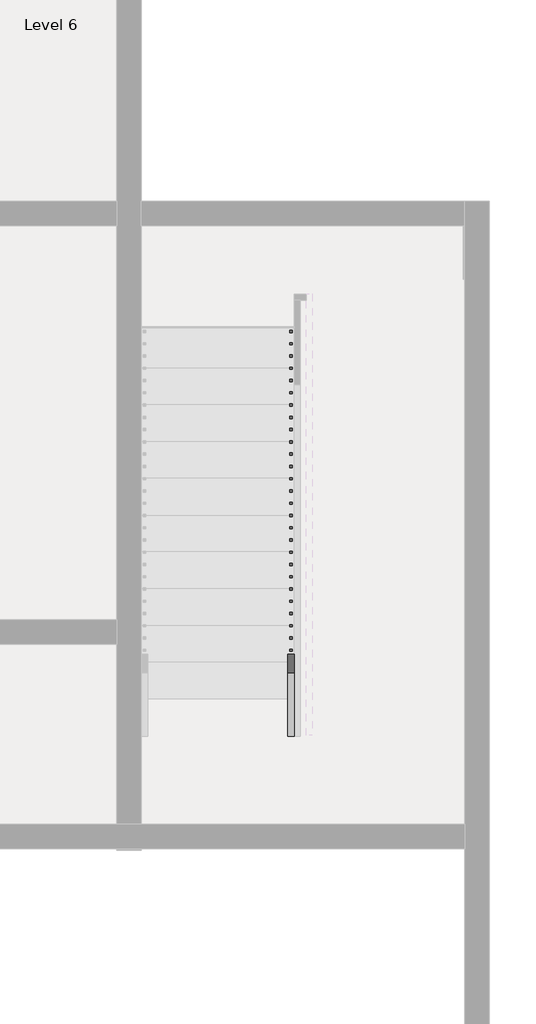
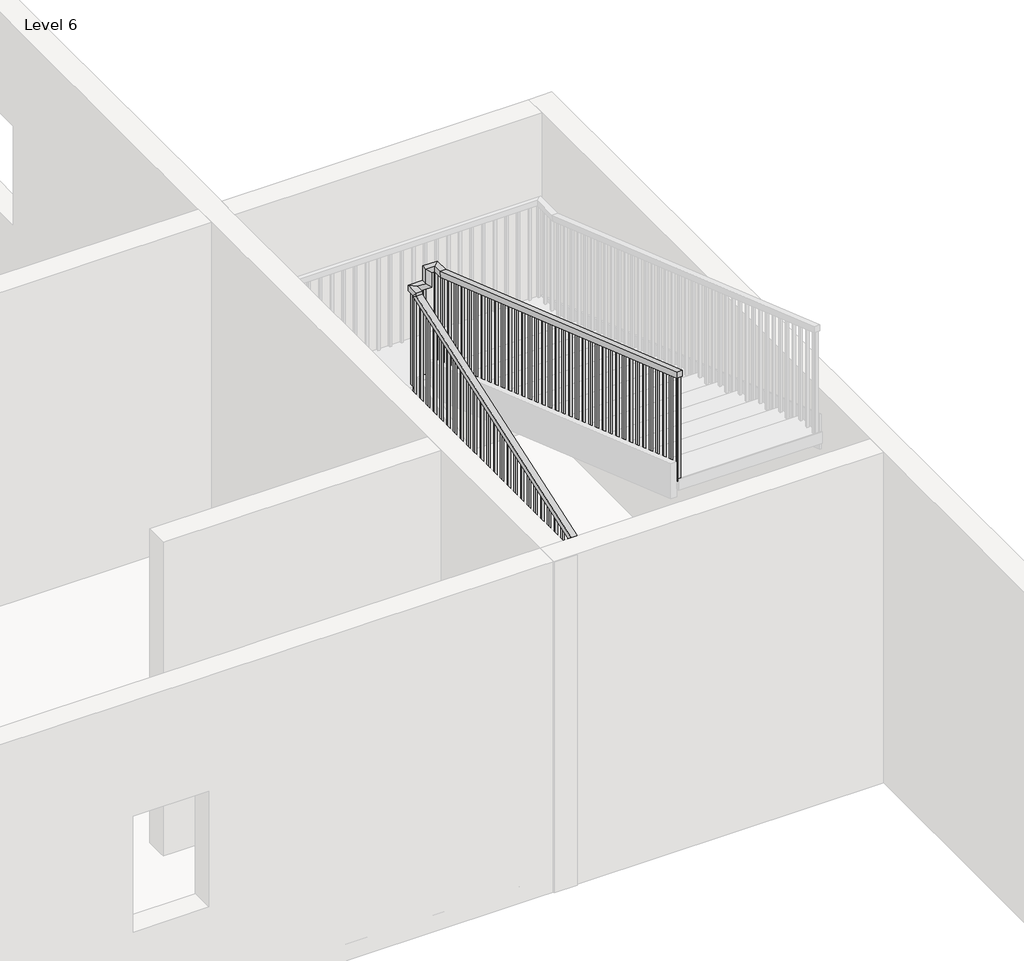
# One storey, part 6 of 14: 1 railing.
"""IFC4 building model written with IfcOpenShell, lengths in millimetres."""

from ifc_helpers import new_model, si_unit, frame, origin, place, context, project, spatial, polyline, outline, extrude, faceted_brep, element, save

model = new_model("IFC4")

# Units and contexts
model_context = context("Model", 3, world=origin())
ifc_project = project(units=[si_unit("LENGTHUNIT", "METRE", prefix="MILLI")], contexts=[model_context])

# Site, building, storey
site = spatial("IfcSite", under=ifc_project)
building = spatial("IfcBuilding", under=site)
storey = spatial("IfcBuildingStorey", under=building, Name="Level 6", Elevation=15240.0)

# Railing
placement = place(None, origin())
element("IfcRailing", 1, ObjectType="Handrail - Rectangular", at=placement, inside=storey, context=model_context, shape_type="SolidModel", body=[
    faceted_brep([(-2644.5381751, -9955.5916506, 16259.9076923), (-2644.5381751, -9955.5916506, 16206.1602476), (-2593.7381751, -9955.5916506, 16206.1602476), (-2593.7381751, -9955.5916506, 16259.9076923), (-2644.5381751, -6367.8416506, 17499.6687908), (-2644.5381751, -6317.0416506, 17463.4754856), (-2593.7381751, -6317.0416506, 17463.4754856), (-2593.7381751, -6367.8416506, 17499.6687908), (-2644.5381751, -6367.8416506, 17526.0), (-2644.5381751, -6317.0416506, 17475.2), (-2593.7381751, -6317.0416506, 17475.2), (-2593.7381751, -6367.8416506, 17526.0), (-2644.5381751, -6240.8416506, 17526.0), (-2644.5381751, -6240.8416506, 17475.2), (-2593.7381751, -6291.6416506, 17475.2), (-2593.7381751, -6291.6416506, 17526.0), (-2517.5381751, -6240.8416506, 17526.0), (-2466.7381751, -6240.8416506, 17475.2), (-2466.7381751, -6291.6416506, 17475.2), (-2517.5381751, -6291.6416506, 17526.0), (-2517.5381751, -6240.8416506, 17657.8846154), (-2466.7381751, -6240.8416506, 17607.0846154), (-2466.7381751, -6291.6416506, 17607.0846154), (-2517.5381751, -6291.6416506, 17657.8846154), (-2390.5381751, -6240.8416506, 17657.8846154), (-2390.5381751, -6240.8416506, 17607.0846154), (-2441.3381751, -6291.6416506, 17607.0846154), (-2441.3381751, -6291.6416506, 17657.8846154), (-2390.5381751, -6367.8416506, 17657.8846154), (-2390.5381751, -6376.3852679, 17607.0846154), (-2441.3381751, -6376.3852679, 17607.0846154), (-2441.3381751, -6367.8416506, 17657.8846154), (-2390.5381751, -9949.2416506, 18897.6), (-2441.3381751, -9949.2416506, 18897.6), (-2441.3381751, -9949.2416506, 18843.842594), (-2390.5381751, -9949.2416506, 18843.842594)], [[[0, 1, 2, 3]], [[1, 0, 4, 5]], [[2, 1, 5, 6]], [[3, 2, 6, 7]], [[0, 3, 7, 4]], [[5, 4, 8, 9]], [[6, 5, 9, 10]], [[7, 6, 10, 11]], [[4, 7, 11, 8]], [[9, 8, 12, 13]], [[10, 9, 13, 14]], [[11, 10, 14, 15]], [[8, 11, 15, 12]], [[13, 12, 16, 17]], [[14, 13, 17, 18]], [[15, 14, 18, 19]], [[12, 15, 19, 16]], [[17, 16, 20, 21]], [[18, 17, 21, 22]], [[19, 18, 22, 23]], [[16, 19, 23, 20]], [[21, 20, 24, 25]], [[22, 21, 25, 26]], [[23, 22, 26, 27]], [[20, 23, 27, 24]], [[25, 24, 28, 29]], [[26, 25, 29, 30]], [[27, 26, 30, 31]], [[24, 27, 31, 28]], [[32, 33, 34, 35]], [[29, 28, 32, 35]], [[30, 29, 35, 34]], [[31, 30, 34, 33]], [[28, 31, 33, 32]]]),
    extrude(outline(polyline([(-9933.3666506, 18838.3474017), (-9914.3166506, 18831.7531709), (-9914.3166506, 17877.6923077), (-9933.3666506, 17877.6923077), (-9933.3666506, 18838.3474017)])), frame((-2425.4631751, 0.0, 0.0), z_axis=(1.0, 0.0, 0.0), x_axis=(0.0, 1.0, 0.0)), (0.0, 0.0, 1.0), 19.05),
    extrude(outline(polyline([(-9831.7666506, 18803.1781709), (-9812.7166506, 18796.5839402), (-9812.7166506, 17877.6923077), (-9831.7666506, 17877.6923077), (-9831.7666506, 18803.1781709)])), frame((-2425.4631751, 0.0, 0.0), z_axis=(1.0, 0.0, 0.0), x_axis=(0.0, 1.0, 0.0)), (0.0, 0.0, 1.0), 19.05),
    extrude(outline(polyline([(-9730.1666506, 18768.0089402), (-9711.1166506, 18761.4147094), (-9711.1166506, 17877.6923077), (-9730.1666506, 17877.6923077), (-9730.1666506, 18768.0089402)])), frame((-2425.4631751, 0.0, 0.0), z_axis=(1.0, 0.0, 0.0), x_axis=(0.0, 1.0, 0.0)), (0.0, 0.0, 1.0), 19.05),
    extrude(outline(polyline([(-9628.5666506, 18732.8397094), (-9609.5166506, 18726.2454786), (-9609.5166506, 17772.1846154), (-9628.5666506, 17772.1846154), (-9628.5666506, 18732.8397094)])), frame((-2425.4631751, 0.0, 0.0), z_axis=(1.0, 0.0, 0.0), x_axis=(0.0, 1.0, 0.0)), (0.0, 0.0, 1.0), 19.05),
    extrude(outline(polyline([(-9526.9666506, 18697.6704786), (-9507.9166506, 18691.0762479), (-9507.9166506, 17772.1846154), (-9526.9666506, 17772.1846154), (-9526.9666506, 18697.6704786)])), frame((-2425.4631751, 0.0, 0.0), z_axis=(1.0, 0.0, 0.0), x_axis=(0.0, 1.0, 0.0)), (0.0, 0.0, 1.0), 19.05),
    extrude(outline(polyline([(-9425.3666506, 18662.5012479), (-9406.3166506, 18655.9070171), (-9406.3166506, 17772.1846154), (-9425.3666506, 17772.1846154), (-9425.3666506, 18662.5012479)])), frame((-2425.4631751, 0.0, 0.0), z_axis=(1.0, 0.0, 0.0), x_axis=(0.0, 1.0, 0.0)), (0.0, 0.0, 1.0), 19.05),
    extrude(outline(polyline([(-9323.7666506, 18627.3320171), (-9304.7166506, 18620.7377863), (-9304.7166506, 17666.6769231), (-9323.7666506, 17666.6769231), (-9323.7666506, 18627.3320171)])), frame((-2425.4631751, 0.0, 0.0), z_axis=(1.0, 0.0, 0.0), x_axis=(0.0, 1.0, 0.0)), (0.0, 0.0, 1.0), 19.05),
    extrude(outline(polyline([(-9222.1666506, 18592.1627863), (-9203.1166506, 18585.5685556), (-9203.1166506, 17666.6769231), (-9222.1666506, 17666.6769231), (-9222.1666506, 18592.1627863)])), frame((-2425.4631751, 0.0, 0.0), z_axis=(1.0, 0.0, 0.0), x_axis=(0.0, 1.0, 0.0)), (0.0, 0.0, 1.0), 19.05),
    extrude(outline(polyline([(-9120.5666506, 18556.9935556), (-9101.5166506, 18550.3993248), (-9101.5166506, 17666.6769231), (-9120.5666506, 17666.6769231), (-9120.5666506, 18556.9935556)])), frame((-2425.4631751, 0.0, 0.0), z_axis=(1.0, 0.0, 0.0), x_axis=(0.0, 1.0, 0.0)), (0.0, 0.0, 1.0), 19.05),
    extrude(outline(polyline([(-9018.9666506, 18521.8243248), (-8999.9166506, 18515.230094), (-8999.9166506, 17561.1692308), (-9018.9666506, 17561.1692308), (-9018.9666506, 18521.8243248)])), frame((-2425.4631751, 0.0, 0.0), z_axis=(1.0, 0.0, 0.0), x_axis=(0.0, 1.0, 0.0)), (0.0, 0.0, 1.0), 19.05),
    extrude(outline(polyline([(-8917.3666506, 18486.655094), (-8898.3166506, 18480.0608632), (-8898.3166506, 17561.1692308), (-8917.3666506, 17561.1692308), (-8917.3666506, 18486.655094)])), frame((-2425.4631751, 0.0, 0.0), z_axis=(1.0, 0.0, 0.0), x_axis=(0.0, 1.0, 0.0)), (0.0, 0.0, 1.0), 19.05),
    extrude(outline(polyline([(-8815.7666506, 18451.4858632), (-8796.7166506, 18444.8916325), (-8796.7166506, 17561.1692308), (-8815.7666506, 17561.1692308), (-8815.7666506, 18451.4858632)])), frame((-2425.4631751, 0.0, 0.0), z_axis=(1.0, 0.0, 0.0), x_axis=(0.0, 1.0, 0.0)), (0.0, 0.0, 1.0), 19.05),
    extrude(outline(polyline([(-8714.1666506, 18416.3166325), (-8695.1166506, 18409.7224017), (-8695.1166506, 17455.6615385), (-8714.1666506, 17455.6615385), (-8714.1666506, 18416.3166325)])), frame((-2425.4631751, 0.0, 0.0), z_axis=(1.0, 0.0, 0.0), x_axis=(0.0, 1.0, 0.0)), (0.0, 0.0, 1.0), 19.05),
    extrude(outline(polyline([(-8612.5666506, 18381.1474017), (-8593.5166506, 18374.5531709), (-8593.5166506, 17455.6615385), (-8612.5666506, 17455.6615385), (-8612.5666506, 18381.1474017)])), frame((-2425.4631751, 0.0, 0.0), z_axis=(1.0, 0.0, 0.0), x_axis=(0.0, 1.0, 0.0)), (0.0, 0.0, 1.0), 19.05),
    extrude(outline(polyline([(-8510.9666506, 18345.9781709), (-8491.9166506, 18339.3839402), (-8491.9166506, 17455.6615385), (-8510.9666506, 17455.6615385), (-8510.9666506, 18345.9781709)])), frame((-2425.4631751, 0.0, 0.0), z_axis=(1.0, 0.0, 0.0), x_axis=(0.0, 1.0, 0.0)), (0.0, 0.0, 1.0), 19.05),
    extrude(outline(polyline([(-8409.3666506, 18310.8089402), (-8390.3166506, 18304.2147094), (-8390.3166506, 17350.1538462), (-8409.3666506, 17350.1538462), (-8409.3666506, 18310.8089402)])), frame((-2425.4631751, 0.0, 0.0), z_axis=(1.0, 0.0, 0.0), x_axis=(0.0, 1.0, 0.0)), (0.0, 0.0, 1.0), 19.05),
    extrude(outline(polyline([(-8307.7666506, 18275.6397094), (-8288.7166506, 18269.0454786), (-8288.7166506, 17350.1538462), (-8307.7666506, 17350.1538462), (-8307.7666506, 18275.6397094)])), frame((-2425.4631751, 0.0, 0.0), z_axis=(1.0, 0.0, 0.0), x_axis=(0.0, 1.0, 0.0)), (0.0, 0.0, 1.0), 19.05),
    extrude(outline(polyline([(-8206.1666506, 18240.4704786), (-8187.1166506, 18233.8762479), (-8187.1166506, 17350.1538462), (-8206.1666506, 17350.1538462), (-8206.1666506, 18240.4704786)])), frame((-2425.4631751, 0.0, 0.0), z_axis=(1.0, 0.0, 0.0), x_axis=(0.0, 1.0, 0.0)), (0.0, 0.0, 1.0), 19.05),
    extrude(outline(polyline([(-8104.5666506, 18205.3012479), (-8085.5166506, 18198.7070171), (-8085.5166506, 17244.6461538), (-8104.5666506, 17244.6461538), (-8104.5666506, 18205.3012479)])), frame((-2425.4631751, 0.0, 0.0), z_axis=(1.0, 0.0, 0.0), x_axis=(0.0, 1.0, 0.0)), (0.0, 0.0, 1.0), 19.05),
    extrude(outline(polyline([(-8002.9666506, 18170.1320171), (-7983.9166506, 18163.5377863), (-7983.9166506, 17244.6461538), (-8002.9666506, 17244.6461538), (-8002.9666506, 18170.1320171)])), frame((-2425.4631751, 0.0, 0.0), z_axis=(1.0, 0.0, 0.0), x_axis=(0.0, 1.0, 0.0)), (0.0, 0.0, 1.0), 19.05),
    extrude(outline(polyline([(-7901.3666506, 18134.9627863), (-7882.3166506, 18128.3685556), (-7882.3166506, 17244.6461538), (-7901.3666506, 17244.6461538), (-7901.3666506, 18134.9627863)])), frame((-2425.4631751, 0.0, 0.0), z_axis=(1.0, 0.0, 0.0), x_axis=(0.0, 1.0, 0.0)), (0.0, 0.0, 1.0), 19.05),
    extrude(outline(polyline([(-7799.7666506, 18099.7935556), (-7780.7166506, 18093.1993248), (-7780.7166506, 17139.1384615), (-7799.7666506, 17139.1384615), (-7799.7666506, 18099.7935556)])), frame((-2425.4631751, 0.0, 0.0), z_axis=(1.0, 0.0, 0.0), x_axis=(0.0, 1.0, 0.0)), (0.0, 0.0, 1.0), 19.05),
    extrude(outline(polyline([(-7698.1666506, 18064.6243248), (-7679.1166506, 18058.030094), (-7679.1166506, 17139.1384615), (-7698.1666506, 17139.1384615), (-7698.1666506, 18064.6243248)])), frame((-2425.4631751, 0.0, 0.0), z_axis=(1.0, 0.0, 0.0), x_axis=(0.0, 1.0, 0.0)), (0.0, 0.0, 1.0), 19.05),
    extrude(outline(polyline([(-7596.5666506, 18029.455094), (-7577.5166506, 18022.8608632), (-7577.5166506, 17139.1384615), (-7596.5666506, 17139.1384615), (-7596.5666506, 18029.455094)])), frame((-2425.4631751, 0.0, 0.0), z_axis=(1.0, 0.0, 0.0), x_axis=(0.0, 1.0, 0.0)), (0.0, 0.0, 1.0), 19.05),
    extrude(outline(polyline([(-7494.9666506, 17994.2858632), (-7475.9166506, 17987.6916325), (-7475.9166506, 17033.6307692), (-7494.9666506, 17033.6307692), (-7494.9666506, 17994.2858632)])), frame((-2425.4631751, 0.0, 0.0), z_axis=(1.0, 0.0, 0.0), x_axis=(0.0, 1.0, 0.0)), (0.0, 0.0, 1.0), 19.05),
    extrude(outline(polyline([(-7393.3666506, 17959.1166325), (-7374.3166506, 17952.5224017), (-7374.3166506, 17033.6307692), (-7393.3666506, 17033.6307692), (-7393.3666506, 17959.1166325)])), frame((-2425.4631751, 0.0, 0.0), z_axis=(1.0, 0.0, 0.0), x_axis=(0.0, 1.0, 0.0)), (0.0, 0.0, 1.0), 19.05),
    extrude(outline(polyline([(-7291.7666506, 17923.9474017), (-7272.7166506, 17917.3531709), (-7272.7166506, 17033.6307692), (-7291.7666506, 17033.6307692), (-7291.7666506, 17923.9474017)])), frame((-2425.4631751, 0.0, 0.0), z_axis=(1.0, 0.0, 0.0), x_axis=(0.0, 1.0, 0.0)), (0.0, 0.0, 1.0), 19.05),
    extrude(outline(polyline([(-7190.1666506, 17888.7781709), (-7171.1166506, 17882.1839402), (-7171.1166506, 16928.1230769), (-7190.1666506, 16928.1230769), (-7190.1666506, 17888.7781709)])), frame((-2425.4631751, 0.0, 0.0), z_axis=(1.0, 0.0, 0.0), x_axis=(0.0, 1.0, 0.0)), (0.0, 0.0, 1.0), 19.05),
    extrude(outline(polyline([(-7088.5666506, 17853.6089402), (-7069.5166506, 17847.0147094), (-7069.5166506, 16928.1230769), (-7088.5666506, 16928.1230769), (-7088.5666506, 17853.6089402)])), frame((-2425.4631751, 0.0, 0.0), z_axis=(1.0, 0.0, 0.0), x_axis=(0.0, 1.0, 0.0)), (0.0, 0.0, 1.0), 19.05),
    extrude(outline(polyline([(-6986.9666506, 17818.4397094), (-6967.9166506, 17811.8454786), (-6967.9166506, 16928.1230769), (-6986.9666506, 16928.1230769), (-6986.9666506, 17818.4397094)])), frame((-2425.4631751, 0.0, 0.0), z_axis=(1.0, 0.0, 0.0), x_axis=(0.0, 1.0, 0.0)), (0.0, 0.0, 1.0), 19.05),
    extrude(outline(polyline([(-6885.3666506, 17783.2704786), (-6866.3166506, 17776.6762479), (-6866.3166506, 16822.6153846), (-6885.3666506, 16822.6153846), (-6885.3666506, 17783.2704786)])), frame((-2425.4631751, 0.0, 0.0), z_axis=(1.0, 0.0, 0.0), x_axis=(0.0, 1.0, 0.0)), (0.0, 0.0, 1.0), 19.05),
    extrude(outline(polyline([(-6783.7666506, 17748.1012479), (-6764.7166506, 17741.5070171), (-6764.7166506, 16822.6153846), (-6783.7666506, 16822.6153846), (-6783.7666506, 17748.1012479)])), frame((-2425.4631751, 0.0, 0.0), z_axis=(1.0, 0.0, 0.0), x_axis=(0.0, 1.0, 0.0)), (0.0, 0.0, 1.0), 19.05),
    extrude(outline(polyline([(-6682.1666506, 17712.9320171), (-6663.1166506, 17706.3377863), (-6663.1166506, 16822.6153846), (-6682.1666506, 16822.6153846), (-6682.1666506, 17712.9320171)])), frame((-2425.4631751, 0.0, 0.0), z_axis=(1.0, 0.0, 0.0), x_axis=(0.0, 1.0, 0.0)), (0.0, 0.0, 1.0), 19.05),
    extrude(outline(polyline([(-6580.5666506, 17677.7627863), (-6561.5166506, 17671.1685556), (-6561.5166506, 16717.1076923), (-6580.5666506, 16717.1076923), (-6580.5666506, 17677.7627863)])), frame((-2425.4631751, 0.0, 0.0), z_axis=(1.0, 0.0, 0.0), x_axis=(0.0, 1.0, 0.0)), (0.0, 0.0, 1.0), 19.05),
    extrude(outline(polyline([(-6478.9666506, 17642.5935556), (-6459.9166506, 17635.9993248), (-6459.9166506, 16717.1076923), (-6478.9666506, 16717.1076923), (-6478.9666506, 17642.5935556)])), frame((-2425.4631751, 0.0, 0.0), z_axis=(1.0, 0.0, 0.0), x_axis=(0.0, 1.0, 0.0)), (0.0, 0.0, 1.0), 19.05),
    extrude(outline(polyline([(-6377.3666506, 17607.4243248), (-6358.3166506, 17600.830094), (-6358.3166506, 16717.1076923), (-6377.3666506, 16717.1076923), (-6377.3666506, 17607.4243248)])), frame((-2425.4631751, 0.0, 0.0), z_axis=(1.0, 0.0, 0.0), x_axis=(0.0, 1.0, 0.0)), (0.0, 0.0, 1.0), 19.05),
    extrude(outline(polyline([(-2527.0631751, -6275.7666506), (-2527.0631751, -6256.7166506), (-2508.0131751, -6256.7166506), (-2508.0131751, -6275.7666506), (-2527.0631751, -6275.7666506)])), frame((0.0, 0.0, 16611.6), z_axis=(0.0, 0.0, 1.0), x_axis=(1.0, 0.0, 0.0)), (0.0, 0.0, 1.0), 863.6),
    extrude(outline(polyline([(-2609.6131751, -6307.5166506), (-2628.6631751, -6307.5166506), (-2628.6631751, -6288.4666506), (-2609.6131751, -6288.4666506), (-2609.6131751, -6307.5166506)])), frame((0.0, 0.0, 16506.0923077), z_axis=(0.0, 0.0, 1.0), x_axis=(1.0, 0.0, 0.0)), (0.0, 0.0, 1.0), 969.1076923),
    extrude(outline(polyline([(-6409.1166506, 17431.6586078), (-6390.0666506, 17438.2414101), (-6390.0666506, 16506.0923077), (-6409.1166506, 16506.0923077), (-6409.1166506, 17431.6586078)])), frame((-2628.6631751, 0.0, 0.0), z_axis=(1.0, 0.0, 0.0), x_axis=(0.0, 1.0, 0.0)), (0.0, 0.0, 1.0), 19.05),
    extrude(outline(polyline([(-6510.7166506, 17396.5503289), (-6491.6666506, 17403.1331312), (-6491.6666506, 16506.0923077), (-6510.7166506, 16506.0923077), (-6510.7166506, 17396.5503289)])), frame((-2628.6631751, 0.0, 0.0), z_axis=(1.0, 0.0, 0.0), x_axis=(0.0, 1.0, 0.0)), (0.0, 0.0, 1.0), 19.05),
    extrude(outline(polyline([(-6612.3166506, 17361.44205), (-6593.2666506, 17368.0248523), (-6593.2666506, 16400.5846154), (-6612.3166506, 16400.5846154), (-6612.3166506, 17361.44205)])), frame((-2628.6631751, 0.0, 0.0), z_axis=(1.0, 0.0, 0.0), x_axis=(0.0, 1.0, 0.0)), (0.0, 0.0, 1.0), 19.05),
    extrude(outline(polyline([(-6713.9166506, 17326.3337711), (-6694.8666506, 17332.9165734), (-6694.8666506, 16400.5846154), (-6713.9166506, 16400.5846154), (-6713.9166506, 17326.3337711)])), frame((-2628.6631751, 0.0, 0.0), z_axis=(1.0, 0.0, 0.0), x_axis=(0.0, 1.0, 0.0)), (0.0, 0.0, 1.0), 19.05),
    extrude(outline(polyline([(-6815.5166506, 17291.2254922), (-6796.4666506, 17297.8082945), (-6796.4666506, 16400.5846154), (-6815.5166506, 16400.5846154), (-6815.5166506, 17291.2254922)])), frame((-2628.6631751, 0.0, 0.0), z_axis=(1.0, 0.0, 0.0), x_axis=(0.0, 1.0, 0.0)), (0.0, 0.0, 1.0), 19.05),
    extrude(outline(polyline([(-6917.1166506, 17256.1172133), (-6898.0666506, 17262.7000156), (-6898.0666506, 16295.0769231), (-6917.1166506, 16295.0769231), (-6917.1166506, 17256.1172133)])), frame((-2628.6631751, 0.0, 0.0), z_axis=(1.0, 0.0, 0.0), x_axis=(0.0, 1.0, 0.0)), (0.0, 0.0, 1.0), 19.05),
    extrude(outline(polyline([(-7018.7166506, 17221.0089344), (-6999.6666506, 17227.5917367), (-6999.6666506, 16295.0769231), (-7018.7166506, 16295.0769231), (-7018.7166506, 17221.0089344)])), frame((-2628.6631751, 0.0, 0.0), z_axis=(1.0, 0.0, 0.0), x_axis=(0.0, 1.0, 0.0)), (0.0, 0.0, 1.0), 19.05),
    extrude(outline(polyline([(-7120.3166506, 17185.9006556), (-7101.2666506, 17192.4834578), (-7101.2666506, 16295.0769231), (-7120.3166506, 16295.0769231), (-7120.3166506, 17185.9006556)])), frame((-2628.6631751, 0.0, 0.0), z_axis=(1.0, 0.0, 0.0), x_axis=(0.0, 1.0, 0.0)), (0.0, 0.0, 1.0), 19.05),
    extrude(outline(polyline([(-7221.9166506, 17150.7923767), (-7202.8666506, 17157.3751789), (-7202.8666506, 16189.5692308), (-7221.9166506, 16189.5692308), (-7221.9166506, 17150.7923767)])), frame((-2628.6631751, 0.0, 0.0), z_axis=(1.0, 0.0, 0.0), x_axis=(0.0, 1.0, 0.0)), (0.0, 0.0, 1.0), 19.05),
    extrude(outline(polyline([(-7323.5166506, 17115.6840978), (-7304.4666506, 17122.2669001), (-7304.4666506, 16189.5692308), (-7323.5166506, 16189.5692308), (-7323.5166506, 17115.6840978)])), frame((-2628.6631751, 0.0, 0.0), z_axis=(1.0, 0.0, 0.0), x_axis=(0.0, 1.0, 0.0)), (0.0, 0.0, 1.0), 19.05),
    extrude(outline(polyline([(-7425.1166506, 17080.5758189), (-7406.0666506, 17087.1586212), (-7406.0666506, 16189.5692308), (-7425.1166506, 16189.5692308), (-7425.1166506, 17080.5758189)])), frame((-2628.6631751, 0.0, 0.0), z_axis=(1.0, 0.0, 0.0), x_axis=(0.0, 1.0, 0.0)), (0.0, 0.0, 1.0), 19.05),
    extrude(outline(polyline([(-7526.7166506, 17045.46754), (-7507.6666506, 17052.0503423), (-7507.6666506, 16084.0615385), (-7526.7166506, 16084.0615385), (-7526.7166506, 17045.46754)])), frame((-2628.6631751, 0.0, 0.0), z_axis=(1.0, 0.0, 0.0), x_axis=(0.0, 1.0, 0.0)), (0.0, 0.0, 1.0), 19.05),
    extrude(outline(polyline([(-7628.3166506, 17010.3592611), (-7609.2666506, 17016.9420634), (-7609.2666506, 16084.0615385), (-7628.3166506, 16084.0615385), (-7628.3166506, 17010.3592611)])), frame((-2628.6631751, 0.0, 0.0), z_axis=(1.0, 0.0, 0.0), x_axis=(0.0, 1.0, 0.0)), (0.0, 0.0, 1.0), 19.05),
    extrude(outline(polyline([(-7729.9166506, 16975.2509822), (-7710.8666506, 16981.8337845), (-7710.8666506, 16084.0615385), (-7729.9166506, 16084.0615385), (-7729.9166506, 16975.2509822)])), frame((-2628.6631751, 0.0, 0.0), z_axis=(1.0, 0.0, 0.0), x_axis=(0.0, 1.0, 0.0)), (0.0, 0.0, 1.0), 19.05),
    extrude(outline(polyline([(-7831.5166506, 16940.1427033), (-7812.4666506, 16946.7255056), (-7812.4666506, 15978.5538462), (-7831.5166506, 15978.5538462), (-7831.5166506, 16940.1427033)])), frame((-2628.6631751, 0.0, 0.0), z_axis=(1.0, 0.0, 0.0), x_axis=(0.0, 1.0, 0.0)), (0.0, 0.0, 1.0), 19.05),
    extrude(outline(polyline([(-7933.1166506, 16905.0344244), (-7914.0666506, 16911.6172267), (-7914.0666506, 15978.5538462), (-7933.1166506, 15978.5538462), (-7933.1166506, 16905.0344244)])), frame((-2628.6631751, 0.0, 0.0), z_axis=(1.0, 0.0, 0.0), x_axis=(0.0, 1.0, 0.0)), (0.0, 0.0, 1.0), 19.05),
    extrude(outline(polyline([(-8034.7166506, 16869.9261455), (-8015.6666506, 16876.5089478), (-8015.6666506, 15978.5538462), (-8034.7166506, 15978.5538462), (-8034.7166506, 16869.9261455)])), frame((-2628.6631751, 0.0, 0.0), z_axis=(1.0, 0.0, 0.0), x_axis=(0.0, 1.0, 0.0)), (0.0, 0.0, 1.0), 19.05),
    extrude(outline(polyline([(-8136.3166506, 16834.8178666), (-8117.2666506, 16841.4006689), (-8117.2666506, 15873.0461538), (-8136.3166506, 15873.0461538), (-8136.3166506, 16834.8178666)])), frame((-2628.6631751, 0.0, 0.0), z_axis=(1.0, 0.0, 0.0), x_axis=(0.0, 1.0, 0.0)), (0.0, 0.0, 1.0), 19.05),
    extrude(outline(polyline([(-8237.9166506, 16799.7095877), (-8218.8666506, 16806.29239), (-8218.8666506, 15873.0461538), (-8237.9166506, 15873.0461538), (-8237.9166506, 16799.7095877)])), frame((-2628.6631751, 0.0, 0.0), z_axis=(1.0, 0.0, 0.0), x_axis=(0.0, 1.0, 0.0)), (0.0, 0.0, 1.0), 19.05),
    extrude(outline(polyline([(-8339.5166506, 16764.6013088), (-8320.4666506, 16771.1841111), (-8320.4666506, 15873.0461538), (-8339.5166506, 15873.0461538), (-8339.5166506, 16764.6013088)])), frame((-2628.6631751, 0.0, 0.0), z_axis=(1.0, 0.0, 0.0), x_axis=(0.0, 1.0, 0.0)), (0.0, 0.0, 1.0), 19.05),
    extrude(outline(polyline([(-8441.1166506, 16729.4930299), (-8422.0666506, 16736.0758322), (-8422.0666506, 15767.5384615), (-8441.1166506, 15767.5384615), (-8441.1166506, 16729.4930299)])), frame((-2628.6631751, 0.0, 0.0), z_axis=(1.0, 0.0, 0.0), x_axis=(0.0, 1.0, 0.0)), (0.0, 0.0, 1.0), 19.05),
    extrude(outline(polyline([(-8542.7166506, 16694.384751), (-8523.6666506, 16700.9675533), (-8523.6666506, 15767.5384615), (-8542.7166506, 15767.5384615), (-8542.7166506, 16694.384751)])), frame((-2628.6631751, 0.0, 0.0), z_axis=(1.0, 0.0, 0.0), x_axis=(0.0, 1.0, 0.0)), (0.0, 0.0, 1.0), 19.05),
    extrude(outline(polyline([(-8644.3166506, 16659.2764721), (-8625.2666506, 16665.8592744), (-8625.2666506, 15767.5384615), (-8644.3166506, 15767.5384615), (-8644.3166506, 16659.2764721)])), frame((-2628.6631751, 0.0, 0.0), z_axis=(1.0, 0.0, 0.0), x_axis=(0.0, 1.0, 0.0)), (0.0, 0.0, 1.0), 19.05),
    extrude(outline(polyline([(-8745.9166506, 16624.1681932), (-8726.8666506, 16630.7509955), (-8726.8666506, 15662.0307692), (-8745.9166506, 15662.0307692), (-8745.9166506, 16624.1681932)])), frame((-2628.6631751, 0.0, 0.0), z_axis=(1.0, 0.0, 0.0), x_axis=(0.0, 1.0, 0.0)), (0.0, 0.0, 1.0), 19.05),
    extrude(outline(polyline([(-8847.5166506, 16589.0599143), (-8828.4666506, 16595.6427166), (-8828.4666506, 15662.0307692), (-8847.5166506, 15662.0307692), (-8847.5166506, 16589.0599143)])), frame((-2628.6631751, 0.0, 0.0), z_axis=(1.0, 0.0, 0.0), x_axis=(0.0, 1.0, 0.0)), (0.0, 0.0, 1.0), 19.05),
    extrude(outline(polyline([(-8949.1166506, 16553.9516354), (-8930.0666506, 16560.5344377), (-8930.0666506, 15662.0307692), (-8949.1166506, 15662.0307692), (-8949.1166506, 16553.9516354)])), frame((-2628.6631751, 0.0, 0.0), z_axis=(1.0, 0.0, 0.0), x_axis=(0.0, 1.0, 0.0)), (0.0, 0.0, 1.0), 19.05),
    extrude(outline(polyline([(-9050.7166506, 16518.8433565), (-9031.6666506, 16525.4261588), (-9031.6666506, 15556.5230769), (-9050.7166506, 15556.5230769), (-9050.7166506, 16518.8433565)])), frame((-2628.6631751, 0.0, 0.0), z_axis=(1.0, 0.0, 0.0), x_axis=(0.0, 1.0, 0.0)), (0.0, 0.0, 1.0), 19.05),
    extrude(outline(polyline([(-9152.3166506, 16483.7350776), (-9133.2666506, 16490.3178799), (-9133.2666506, 15556.5230769), (-9152.3166506, 15556.5230769), (-9152.3166506, 16483.7350776)])), frame((-2628.6631751, 0.0, 0.0), z_axis=(1.0, 0.0, 0.0), x_axis=(0.0, 1.0, 0.0)), (0.0, 0.0, 1.0), 19.05),
    extrude(outline(polyline([(-9253.9166506, 16448.6267987), (-9234.8666506, 16455.209601), (-9234.8666506, 15556.5230769), (-9253.9166506, 15556.5230769), (-9253.9166506, 16448.6267987)])), frame((-2628.6631751, 0.0, 0.0), z_axis=(1.0, 0.0, 0.0), x_axis=(0.0, 1.0, 0.0)), (0.0, 0.0, 1.0), 19.05),
    extrude(outline(polyline([(-9355.5166506, 16413.5185198), (-9336.4666506, 16420.1013221), (-9336.4666506, 15451.0153846), (-9355.5166506, 15451.0153846), (-9355.5166506, 16413.5185198)])), frame((-2628.6631751, 0.0, 0.0), z_axis=(1.0, 0.0, 0.0), x_axis=(0.0, 1.0, 0.0)), (0.0, 0.0, 1.0), 19.05),
    extrude(outline(polyline([(-9457.1166506, 16378.4102409), (-9438.0666506, 16384.9930432), (-9438.0666506, 15451.0153846), (-9457.1166506, 15451.0153846), (-9457.1166506, 16378.4102409)])), frame((-2628.6631751, 0.0, 0.0), z_axis=(1.0, 0.0, 0.0), x_axis=(0.0, 1.0, 0.0)), (0.0, 0.0, 1.0), 19.05),
    extrude(outline(polyline([(-9558.7166506, 16343.301962), (-9539.6666506, 16349.8847643), (-9539.6666506, 15451.0153846), (-9558.7166506, 15451.0153846), (-9558.7166506, 16343.301962)])), frame((-2628.6631751, 0.0, 0.0), z_axis=(1.0, 0.0, 0.0), x_axis=(0.0, 1.0, 0.0)), (0.0, 0.0, 1.0), 19.05),
    extrude(outline(polyline([(-9660.3166506, 16308.1936831), (-9641.2666506, 16314.7764854), (-9641.2666506, 15345.5076923), (-9660.3166506, 15345.5076923), (-9660.3166506, 16308.1936831)])), frame((-2628.6631751, 0.0, 0.0), z_axis=(1.0, 0.0, 0.0), x_axis=(0.0, 1.0, 0.0)), (0.0, 0.0, 1.0), 19.05),
    extrude(outline(polyline([(-9761.9166506, 16273.0854043), (-9742.8666506, 16279.6682065), (-9742.8666506, 15345.5076923), (-9761.9166506, 15345.5076923), (-9761.9166506, 16273.0854043)])), frame((-2628.6631751, 0.0, 0.0), z_axis=(1.0, 0.0, 0.0), x_axis=(0.0, 1.0, 0.0)), (0.0, 0.0, 1.0), 19.05),
    extrude(outline(polyline([(-9863.5166506, 16237.9771254), (-9844.4666506, 16244.5599277), (-9844.4666506, 15345.5076923), (-9863.5166506, 15345.5076923), (-9863.5166506, 16237.9771254)])), frame((-2628.6631751, 0.0, 0.0), z_axis=(1.0, 0.0, 0.0), x_axis=(0.0, 1.0, 0.0)), (0.0, 0.0, 1.0), 19.05),
    extrude(outline(polyline([(-2425.4631751, -6275.7666506), (-2425.4631751, -6256.7166506), (-2406.4131751, -6256.7166506), (-2406.4131751, -6275.7666506), (-2425.4631751, -6275.7666506)])), frame((0.0, 0.0, 16611.6), z_axis=(0.0, 0.0, 1.0), x_axis=(1.0, 0.0, 0.0)), (0.0, 0.0, 1.0), 995.4846154),
    extrude(outline(polyline([(-2609.6131751, -6275.7666506), (-2628.6631751, -6275.7666506), (-2628.6631751, -6256.7166506), (-2609.6131751, -6256.7166506), (-2609.6131751, -6275.7666506)])), frame((0.0, 0.0, 16611.6), z_axis=(0.0, 0.0, 1.0), x_axis=(1.0, 0.0, 0.0)), (0.0, 0.0, 1.0), 863.6),
    extrude(outline(polyline([(-9949.2416506, 18843.842594), (-9930.1916506, 18837.2483632), (-9930.1916506, 17877.6923077), (-9949.2416506, 17877.6923077), (-9949.2416506, 18843.842594)])), frame((-2425.4631751, 0.0, 0.0), z_axis=(1.0, 0.0, 0.0), x_axis=(0.0, 1.0, 0.0)), (0.0, 0.0, 1.0), 19.05),
    extrude(outline(polyline([(-9955.5916506, 16206.1602476), (-9936.5416506, 16212.7430499), (-9936.5416506, 15345.5076923), (-9955.5916506, 15345.5076923), (-9955.5916506, 16206.1602476)])), frame((-2628.6631751, 0.0, 0.0), z_axis=(1.0, 0.0, 0.0), x_axis=(0.0, 1.0, 0.0)), (0.0, 0.0, 1.0), 19.05),
])

save(model, "model.ifc")

# Revit data of these elements
# Type "Handrail - Rectangular"
#   Assembly Code = "C2010400"
#   built-in parameter 1008612 = 0.0416667 (stored number, unit not read)
#   built-in parameter 1008611 = 0.0416667 (stored number, unit not read)
#   built-in parameter 1008609 = 0.333333 (stored number, unit not read)
#   built-in parameter 1008604 = 0.166667 (stored number, unit not read)
#   built-in parameter 1008603 = 0.166667 (stored number, unit not read)
#   Railing Height = 3' - 0"
#   built-in parameter 1008630 = 2
#   built-in parameter 1008610 = 2
#   built-in parameter 1008618 = Baluster - Square : 3/4"
# Element 1 (IfcRailing, "Handrail - Rectangular")
#   Phase Created = New Construction
